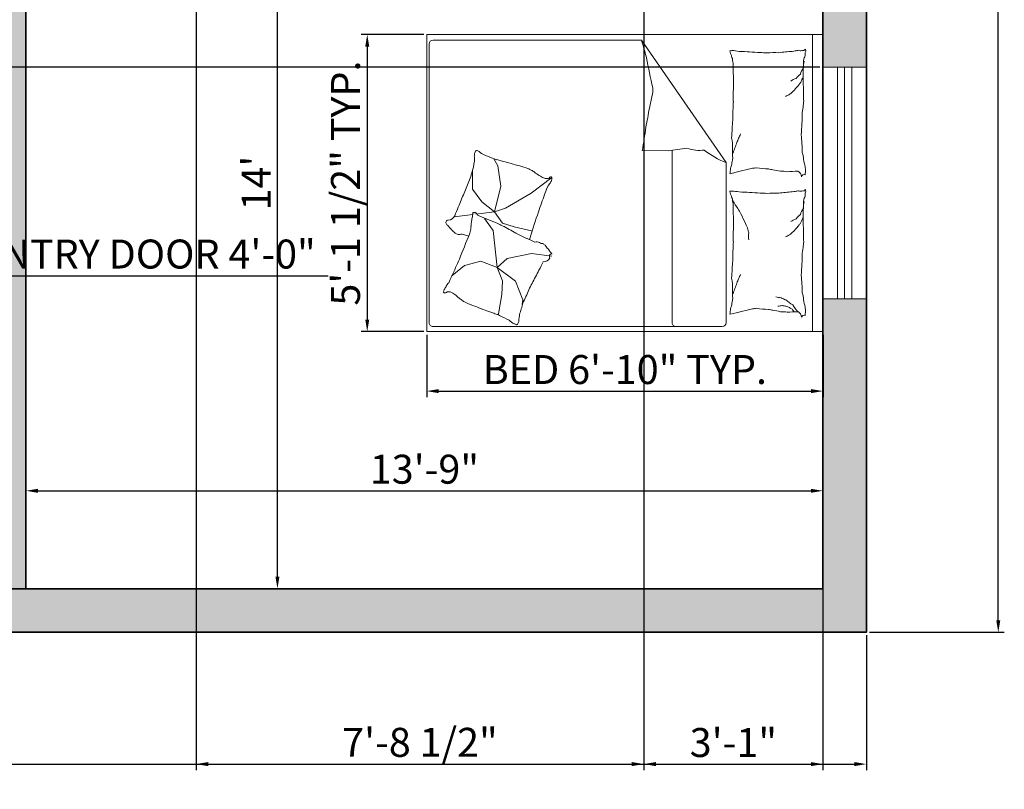
# Model space of a CAD drawing. Units: inches. Extents: x -40 to 424, y -33 to 568.
# Tile 2 of 8: x 209 to 413, y -33 to 127. Entities that reach past the tile are written whole.
import ezdxf

# ---------------------------------------------------------------- set-up
doc = ezdxf.new("R2010")
doc.units = ezdxf.units.IN
for name, color, linetype, lineweight in [('A-ANNO-DIMS', 7, 'Continuous', 18), ('A-FURN', 7, 'Continuous', 18), ('A-GLAZ', 7, 'Continuous', 18), ('A-WALL-PATT', 30, 'Continuous', 13), ('wall', 7, 'Continuous', 35)]:
    doc.layers.add(name, color=color, linetype=linetype, lineweight=lineweight)
doc.styles.add('DIM_FONT', font='SIMPLEX.shx', dxfattribs={"width": 0.8})
doc.styles.get("Standard").update_dxf_attribs({"font": 'arial.ttf'})
doc.dimstyles.new('ISO-25', dxfattribs={"dimtxt": 6, "dimasz": 2.5, "dimexe": 1.25, "dimexo": 0.625, "dimtad": 1, "dimdec": 1, "dimlunit": 3, "dimtxsty": 'Standard', "dimcen": 2.5, "dimadec": 0, "dimazin": 0, "dimtfac": 1, "dimtdec": 1, "dimtmove": 0, "dimatfit": 3, "dimfxl": 1, "dimarcsym": 0})

# ---------------------------------------------------------------- blocks, each defined once
blk = doc.blocks.new('A$C79B528CE')
for p, q in [((1.5, 2), (0, 2)), ((0, 2), (0, 0)), ((1.5, 0), (1.5, 2)), ((1.5, 1.9476), (0, 1.9476)), ((0.6954, 1.5617), (0.6748, 1.6443)), ((1.4047, 1.5617), (1.384, 1.6443)), ((0.7029, 1.5317), (0.6954, 1.5617)), ((1.4122, 1.5317), (1.4047, 1.5617)), ((0.6465, 1.5115), (0.0284, 1.0841)), ((0.6465, 1.5115), (1.4542, 1.5115)), ((1.4742, 1.4915), (1.4742, 0.0322)), ((0.574, 1.3138), (0.5876, 1.2184)), ((1.4542, 1.2389), (0.5847, 1.2389)), ((0.5876, 1.2184), (0.5859, 1.0883)), ((0.0284, 0.0322), (0.0284, 1.0841)), ((0.7224, 0.6316), (0.8016, 0.5276)), ((1.119, 0.6317), (1.1052, 0.5286)), ((0.8016, 0.5276), (0.8767, 0.3973)), ((0.9716, 0.4407), (0.9914, 0.5296)), ((1.1052, 0.5286), (1.131, 0.4065)), ((1.1757, 0.355), (1.2446, 0.4478)), ((1.2446, 0.4478), (1.3392, 0.4856)), ((1.3392, 0.4856), (1.3632, 0.4822)), ((0.9518, 0.3834), (0.9716, 0.4407)), ((1.131, 0.4065), (1.1757, 0.355)), ((0.6632, 0.3597), (0.6272, 0.3397)), ((0.766, 0.3736), (0.6632, 0.3597)), ((0.8945, 0.342), (0.766, 0.3736)), ((0.8767, 0.3973), (0.8945, 0.342)), ((0.8945, 0.342), (0.9518, 0.3834)), ((0.9527, 0.3558), (0.9297, 0.2995)), ((1.1757, 0.355), (0.99, 0.3361)), ((1.1757, 0.355), (1.1448, 0.2725)), ((1.1757, 0.355), (1.2428, 0.3825)), ((1.2428, 0.3825), (1.3116, 0.379)), ((1.3116, 0.379), (1.4097, 0.3619)), ((1.4097, 0.3619), (1.413, 0.3554)), ((0.8945, 0.342), (0.8451, 0.2787)), ((0.8945, 0.342), (0.9063, 0.2478)), ((0.9297, 0.2995), (0.9119, 0.256)), ((0.9401, 0.3), (0.928, 0.2914)), ((0.99, 0.3361), (0.9401, 0.3)), ((0.8451, 0.2787), (0.7799, 0.2313)), ((1.1448, 0.2725), (1.1654, 0.19)), ((0.7799, 0.2313), (0.687, 0.2313)), ((0.9081, 0.2331), (0.92, 0.1385)), ((1.1654, 0.19), (1.219, 0.1274)), ((1.4542, 0.0122), (0.0484, 0.0122)), ((0, 0), (1.5, 0))]:
    blk.add_line(p, q)
for centre, radius, start, end in [((0.0726, 1.9139), 0.00342, 291.7883, 340.436), ((0.0743, 1.9085), 0.00232, 340.436, 101.8931), ((0.0739, 1.9378), 0.0251, 274.3025, 291.7883), ((0.0805, 1.9093), 0.00428, 201.9904, 281.8931), ((0.049, 1.8889), 0.0328, 338.579, 8.1335), ((0.0959, 1.8994), 0.0156, 158.579, 201.9904), ((0.098, 1.9393), 0.0289, 239.3487, 274.3025), ((0.0952, 1.8568), 0.0539, 59.3487, 84.7408), ((0.0953, 1.0829), 0.8208, 84.7408, 88.0921), ((0.1612, 2.0005), 0.0992, 254.0648, 274.2159), ((0.2269, 1.9817), 0.0992, 233.9136, 254.0648), ((0.1856, 0.406), 1.4943, 88.0921, 90.5757), ((0.323, 2.1075), 0.234, 242.7604, 249.1397), ((0.3084, 1.0293), 0.8732, 90.5757, 94.8018), ((0.2874, 1.949), 0.0768, 231.6114, 242.7604), ((0.3125, 2.1919), 0.2897, 267.4614, 274.8018), ((0.3637, 2.0532), 0.1524, 259.8101, 267.4614), ((0.3008, 1.3747), 0.5293, 79.8101, 83.9133), ((0.3945, 0.8466), 1.049, 83.9133, 90), ((0.5954, 1.2129), 0.6827, 90, 97.5469), ((0.6611, 1.6625), 0.2422, 97.5469, 105.744), ((0.5846, 2.2041), 0.3048, 278.4372, 285.744), ((0.6672, 2.0719), 0.1611, 270, 278.4372), ((0.7204, 1.8579), 0.0342, 94.4002, 153.4195), ((0.7086, 2.0011), 0.0904, 258.7276, 270), ((0.7203, 1.9049), 0.0131, 153.4195, 258.7276), ((0.7818, 1.9139), 0.00342, 291.7883, 340.436), ((0.7836, 1.9085), 0.00232, 340.436, 101.8931), ((0.7831, 1.9378), 0.0251, 274.3025, 291.7883), ((0.7897, 1.9093), 0.00428, 201.9904, 281.8931), ((0.7582, 1.8889), 0.0328, 338.579, 8.1335), ((0.8051, 1.8994), 0.0156, 158.579, 201.9904), ((0.8072, 1.9393), 0.0289, 239.3487, 274.3025), ((0.8044, 1.8568), 0.0539, 59.3487, 84.7408), ((0.8046, 1.0829), 0.8208, 84.7408, 88.0921), ((0.8704, 2.0005), 0.0992, 254.0648, 274.2159), ((0.9361, 1.9817), 0.0992, 233.9136, 254.0648), ((0.8948, 0.406), 1.4943, 88.0921, 90.5757), ((1.0323, 2.1075), 0.234, 242.7604, 249.1397), ((1.0177, 1.0293), 0.8732, 90.5757, 94.8018), ((0.9966, 1.949), 0.0768, 231.6114, 242.7604), ((1.0217, 2.1919), 0.2897, 267.4614, 274.8018), ((1.0729, 2.0532), 0.1524, 259.8101, 267.4614), ((1.0101, 1.3747), 0.5293, 79.8101, 83.9133), ((1.1037, 0.8466), 1.049, 83.9133, 90), ((1.3046, 1.2129), 0.6827, 90, 97.5469), ((1.3703, 1.6625), 0.2422, 97.5469, 105.744), ((1.2938, 2.2041), 0.3048, 278.4372, 285.744), ((1.3765, 2.0719), 0.1611, 270, 278.4372), ((1.4296, 1.8579), 0.0342, 94.4002, 153.4195), ((1.4178, 2.0011), 0.0904, 258.7276, 270), ((1.4295, 1.9049), 0.0131, 153.4195, 258.7276), ((-0.1611, 1.8253), 0.246, 8.1335, 12.1095), ((0.279, 1.8867), 0.1983, 187.6809, 192.1095), ((0.9966, 1.8987), 0.9131, 183.3687, 187.6809), ((0.2797, 1.9449), 0.0992, 216.1766, 233.9136), ((0.3154, 1.8961), 0.0992, 198.4397, 216.1766), ((0.5234, 2.1633), 0.3916, 226.1885, 231.6114), ((0.4551, 1.9982), 0.2252, 219.0349, 226.1885), ((1.1818, 1.8735), 0.4918, 180, 186.2324), ((0.5482, 1.8253), 0.246, 8.1335, 12.1095), ((0.9883, 1.8867), 0.1983, 187.6809, 192.1095), ((1.7058, 1.8987), 0.9131, 183.3687, 187.6809), ((0.989, 1.9449), 0.0992, 216.1766, 233.9136), ((1.0247, 1.8961), 0.0992, 198.4397, 216.1766), ((1.2326, 2.1633), 0.3916, 226.1885, 231.6114), ((1.1643, 1.9982), 0.2252, 219.0349, 226.1885), ((1.2401, 1.9123), 0.1399, 314.9024, 332.6012), ((1.3004, 1.9723), 0.1399, 297.2036, 314.9024), ((1.3389, 1.8667), 0.0526, 318.5571, 334.6449), ((1.3333, 1.9167), 0.0899, 306.2641, 318.5571), ((1.891, 1.8735), 0.4918, 180, 186.2324), ((0.3426, 1.8591), 0.0493, 208.3168, 219.0349), ((0.4886, 1.9062), 0.2002, 203.0028, 208.3168), ((0.8939, 1.7858), 0.204, 170.3156, 180), ((1.0518, 1.8591), 0.0493, 208.3168, 219.0349), ((1.1978, 1.9062), 0.2002, 203.0028, 208.3168), ((1.2048, 1.8529), 0.1399, 332.6012, 343.485), ((1.3147, 1.8132), 0.0562, 341.2201, 0), ((1.2793, 1.7719), 0.0915, 0, 14.6851), ((1.18, 1.8895), 0.2056, 338.1851, 341.2201), ((1.2381, 1.8881), 0.1511, 334.6449, 338.1851), ((1.6031, 1.7858), 0.204, 170.3156, 180), ((0.7702, 1.7573), 0.6787, 178.3669, 183.3687), ((0.3686, 1.792), 0.3171, 347.8016, 351.9949), ((1.552, 1.5994), 0.882, 167.8016, 170.3156), ((1.4794, 1.7573), 0.6787, 178.3669, 183.3687), ((1.1897, 1.8023), 0.1399, 343.485, 354.3689), ((1.0778, 1.792), 0.3171, 347.8016, 351.9949), ((2.2613, 1.5994), 0.882, 167.8016, 170.3156), ((1.4559, 1.6447), 1.3652, 176.945, 178.3669), ((0.0204, 1.7556), 0.6588, 351.9949, 357.3351), ((2.1651, 1.6447), 1.3652, 176.945, 178.3669), ((0.7297, 1.7556), 0.6588, 351.9949, 357.3351), ((13.7013, 0.85), 13.6356, 176.49514, 176.94504), ((0.6071, 1.6474), 0.0677, 357.3351, 14.0452), ((14.4105, 0.85), 13.6356, 176.49514, 176.94504), ((1.3164, 1.6474), 0.0677, 357.3351, 14.0452), ((0.3151, 2.8912), 1.4323, 294.3265, 296.4985), ((0.7753, 2.0834), 0.5066, 290.6743, 294.3265), ((0.9799, 1.6796), 0.058, 274.0828, 290.6743), ((1.0172, 1.8969), 0.2721, 266.4448, 274.0828), ((0.4014, 1.5209), 0.3212, 170.0016, 176.4951), ((0.1, 1.5832), 0.0453, 282.869, 297.2841), ((0.1117, 1.6885), 0.1459, 273.574, 282.869), ((0.1384, 2.7103), 1.164, 270.2865, 273.574), ((0.3078, 7.2662), 5.7185, 269.0296, 270.2865), ((0.4895, 4.9065), 3.3622, 267.3904, 269.0296), ((0.5304, 2.7573), 1.2165, 265.3824, 267.3904), ((0.4077, 0.139), 1.4048, 85.3824, 87.2509), ((0.2076, 0.9067), 0.7387, 64.6889, 66.5156), ((0.5669, 1.3138), 0.2301, 87.2509, 101.5586), ((0.2508, 0.888), 0.7387, 66.5156, 68.3423), ((0.2995, 0.8688), 0.7387, 68.3423, 70.572), ((0.3537, 0.8497), 0.7387, 70.572, 72.8018), ((0.5943, 1.6886), 0.1459, 263.5659, 281.5586), ((0.6593, 1.6599), 0.1197, 252.6136, 263.5659), ((0.608, 1.3144), 0.2297, 72.6136, 80.5159), ((1.1107, 1.5209), 0.3212, 170.0016, 176.4951), ((0.8093, 1.5832), 0.0453, 282.869, 297.2841), ((0.8209, 1.6885), 0.1459, 273.574, 282.869), ((0.4519, 2.1618), 0.7286, 302.135, 305.8263), ((0.8476, 2.7103), 1.164, 270.2865, 273.574), ((0.7388, 1.8508), 0.3126, 296.4985, 302.135), ((1.017, 7.2662), 5.7185, 269.0296, 270.2865), ((1.1987, 4.9065), 3.3622, 267.3904, 269.0296), ((1.2397, 2.7573), 1.2165, 265.3824, 267.3904), ((1.1169, 0.139), 1.4048, 85.3824, 87.2509), ((0.9169, 0.9067), 0.7387, 64.6889, 66.5156), ((1.2761, 1.3138), 0.2301, 87.2509, 101.5586), ((0.9601, 0.888), 0.7387, 66.5156, 68.3423), ((1.0087, 0.8688), 0.7387, 68.3423, 70.572), ((1.0629, 0.8497), 0.7387, 70.572, 72.8018), ((1.3035, 1.6886), 0.1459, 263.5659, 281.5586), ((1.3685, 1.6599), 0.1197, 252.6136, 263.5659), ((1.3172, 1.3144), 0.2297, 72.6136, 80.5159), ((0.0623, 1.535), 0.0193, 350.0016, 16.6978), ((0.0815, 1.5304), 0.00132, 16.6978, 97.1204), ((0.1072, 1.4467), 0.0875, 97.1204, 106.2212), ((0.1315, 1.4654), 0.0767, 106.2212, 117.2841), ((0.2944, 1.6407), 0.3751, 320.3555, 339.8512), ((0.6574, 1.2635), 0.2708, 80.5159, 85.9171), ((0.7029, 1.5308), 0.000917, 85.9171, 194.0449), ((0.7716, 1.535), 0.0193, 350.0016, 16.6978), ((0.7908, 1.5304), 0.00132, 16.6978, 97.1204), ((0.8165, 1.4467), 0.0875, 97.1204, 106.2212), ((0.8408, 1.4654), 0.0767, 106.2212, 117.2841), ((1.3666, 1.2635), 0.2708, 80.5159, 85.9171), ((1.4121, 1.5308), 0.000917, 85.9171, 194.0449), ((1.4542, 1.4915), 0.02, 0, 90), ((0.4049, 1.3759), 0.1801, 339.8512, 8.1356), ((1.4542, 1.2589), 0.02, 270, 0), ((-0.4754, 2.8487), 1.8351, 285.9352, 287.7364), ((-0.0634, 1.7415), 0.6574, 282.9255, 285.9352), ((-0.6395, 5.1029), 4.0646, 280.7276, 282.9255), ((0.2775, 1.1989), 0.0581, 262.2696, 280.7276), ((0.3326, 1.3309), 0.1942, 256.8096, 262.2696), ((-0.2025, -1.3253), 2.5158, 76.8096, 78.3259), ((-0.0554, -1.4284), 2.588, 78.3259, 80.505), ((-0.0377, -2.64), 3.7801, 80.505, 82.308), ((0.7246, 0.6267), 0.0063, 166.7192, 233.4208), ((0.7227, 0.6272), 0.00443, 93.9484, 166.7192), ((0.7124, 0.6103), 0.0142, 10.4074, 53.4208), ((0.7249, 0.5964), 0.0352, 69.6548, 93.9484), ((0.6889, 0.6079), 0.0393, 333.1821, 345.4291), ((0.6504, 0.5989), 0.0771, 2.7286, 10.4074), ((0.7122, 0.6019), 0.0153, 345.4291, 2.7286), ((0.7162, 0.5731), 0.0601, 51.4146, 69.6548), ((0.8031, 0.682), 0.0792, 231.4146, 247.2931), ((1.0957, 1.3811), 0.8371, 247.2931, 249.8713), ((1.0012, 0.6426), 0.0774, 313.5224, 324.1064), ((0.9323, 0.7705), 0.2176, 307.2151, 313.5224), ((0.692, 1.1456), 0.6605, 306.2163, 307.2151), ((1.3244, 0.3162), 0.3825, 126.2163, 127.5287), ((1.1299, 0.5924), 0.0452, 127.5287, 134.1274), ((1.0587, 0.6825), 0.0697, 308.8136, 314.1274), ((1.1199, 0.6318), 0.0127, 176.7545, 308.8136), ((1.1115, 0.59), 0.0359, 356.7545, 62.7098), ((0.5455, 0.6678), 0.194, 320.2995, 329.0944), ((0.4099, 0.749), 0.352, 329.0944, 333.1821), ((2.5607, 5.3783), 5.0942, 249.8713, 250.9164), ((1.9234, 3.5362), 3.145, 250.9164, 253.3915), ((1.0928, 0.5526), 0.0458, 157.5838, 188.0492), ((1.0322, 0.5833), 0.0226, 324.1064, 8.0492), ((-0.2306, -2.1858), 3.0972, 62.7098, 63.5853), ((2.1205, 2.3551), 2.0162, 242.5001, 243.5853), ((4.0739, 5.9445), 6.1019, 242.15178, 242.50014), ((2.5804, -0.112), 2.003, 162.1604, 164.7375), ((0.8608, 0.4414), 0.1965, 153.9265, 162.1604), ((0.7571, 0.4922), 0.081, 140.2995, 153.9265), ((2.5307, -0.2643), 1.6868, 152.9116, 154.9471), ((1.0578, 0.6341), 0.1166, 253.3915, 259.2634), ((1.9583, 0.1204), 1.0054, 154.9471, 157.5838), ((-1.4387, -4.647), 5.8383, 62.15178, 62.50792), ((1.0676, -0.068), 0.6236, 62.5079, 69.2514), ((2.3589, -0.3311), 1.5652, 150.064, 152.9116), ((1.2615, 0.0657), 0.43, 69.2514, 77.3748), ((1.4175, 0.4049), 0.063, 77.3748, 93.3881), ((1.4448, 0.5247), 0.0599, 256.9598, 273.3881), ((1.4751, 0.5082), 0.0509, 238.3083, 256.9598), ((1.4772, 0.441), 0.0168, 130.5086, 180.9614), ((1.4694, 0.4587), 0.0058, 180.9614, 238.3083), ((2.2381, -0.0186), 1.6481, 164.7375, 166.159), ((-0.9672, 1.5491), 2.6619, 333.6668, 334.8268), ((1.3928, 0.4743), 0.0755, 310.5086, 333.6668), ((0.4592, 0.4035), 0.1798, 339.2227, 343.6878), ((0.1082, 0.5062), 0.5454, 343.6878, 346.159), ((0.767, 0.4627), 0.2143, 330.064, 337.7645), ((0.895, 0.5261), 0.5454, 339.2919, 341.7631), ((1.2503, 0.4319), 0.1798, 334.8268, 339.2919), ((-1.8615, 1.284), 2.6619, 338.0627, 339.2227), ((2.9572, -0.2212), 1.6481, 160.3416, 161.7631), ((0.6027, 0.2524), 0.0168, 134.9045, 185.3572), ((0.5918, 0.2513), 0.0058, 185.3572, 242.7041), ((0.5376, 0.3177), 0.0755, 314.9045, 338.0627), ((0.9188, 0.234), 0.0231, 107.1867, 157.7645), ((3.2459, -0.4634), 2.003, 157.7645, 160.3416), ((0.6125, 0.2914), 0.0509, 242.7041, 261.3557), ((0.6138, 0.3003), 0.0599, 261.3557, 277.784), ((0.6305, 0.1786), 0.063, 81.7707, 97.784), ((0.5779, -0.1846), 0.43, 73.6473, 81.7707), ((0.5234, -0.3705), 0.6236, 66.9038, 73.6473), ((-1.5222, -5.1672), 5.8383, 66.54766, 66.9038), ((0.8959, 0.2383), 0.00467, 287.1867, 70.6201), ((0.8979, 0.2247), 0.0092, 70.6201, 94.2593), ((0.9057, 0.267), 0.034, 262.0178, 274.2593), ((0.9584, 0.4221), 0.1955, 255.1193, 262.0178), ((0.9073, 0.0507), 0.1794, 75.1193, 82.3216), ((0.959, 0.153), 0.0712, 82.3216, 94.5118), ((0.9779, 0.2893), 0.0663, 261.8784, 274.5118), ((1.0249, 0.332), 0.1166, 248.9957, 261.8784), ((2.2614, 3.1012), 3.145, 246.5205, 248.9957), ((1.9669, -0.1202), 1.0054, 160.6552, 161.9797), ((1.529, 0.1108), 0.1965, 149.5306, 157.7645), ((3.2298, 5.7866), 6.1019, 246.54766, 246.89602), ((1.6266, 2.0287), 2.0162, 246.896, 247.9812), ((-0.2904, -2.7118), 3.0972, 67.1056, 67.9812), ((0.9408, 0.1905), 0.0774, 317.9183, 328.5023), ((0.9875, 0.1619), 0.0226, 328.5023, 12.4451), ((1.0543, 0.1766), 0.0458, 161.9797, 192.4451), ((3.2487, 4.7998), 5.0942, 245.4754, 246.5205), ((1.1772, 0.2819), 0.194, 315.9036, 324.6985), ((1.4053, 0.1288), 0.081, 135.9036, 149.5306), ((0.9005, 0.1084), 0.0359, 1.1504, 67.1056), ((0.9491, 0.1094), 0.0127, 181.1504, 313.2095), ((0.9101, 0.1509), 0.0697, 313.2095, 318.5233), ((0.9962, 0.0748), 0.0452, 131.9246, 138.5233), ((1.2216, -0.1762), 0.3825, 130.6122, 131.9246), ((0.5426, 0.6156), 0.6605, 310.6122, 311.611), ((0.8367, 0.2845), 0.2176, 311.611, 317.9183), ((1.6004, 0.8725), 0.8371, 242.8972, 245.4754), ((1.3069, 0.1689), 0.0792, 227.0187, 242.8972), ((1.2839, 0.1188), 0.0153, 341.0332, 358.3327), ((1.2216, 0.1058), 0.0771, 358.3327, 6.0115), ((1.2895, 0.0928), 0.0142, 6.0115, 49.0249), ((1.2655, 0.1388), 0.0393, 328.7862, 341.0332), ((1.0155, 0.3294), 0.352, 324.6985, 328.7862), ((1.2457, 0.0438), 0.0601, 47.0187, 65.2589), ((1.2864, 0.0526), 0.0352, 65.2589, 89.5525), ((1.3054, 0.0832), 0.00443, 89.5525, 162.3233), ((1.3095, 0.0924), 0.0063, 162.3233, 229.0249), ((0.0484, 0.0322), 0.02, 180, 270), ((1.4542, 0.0322), 0.02, 270, 0)]:
    blk.add_arc(centre, radius, start, end)
at = {"style": 'DIM_FONT', "oblique": -180, "text_generation_flag": 4, "width": 0.8, "flags": 9}
for tag in ['XSIZE', 'YSIZE']:
    blk.add_attdef(tag, (1.5, 2), '', height=0.0005, rotation=180, dxfattribs=at)
blk = doc.blocks.new('*D19')
at = {"layer": 'A-ANNO-DIMS', "color": 0, "lineweight": -2, "transparency": 16777216}
for p, q in [((210, 26.12), (210, 30.54)), ((212.5, 29.29), (372.5, 29.29)), ((375, 26.12), (375, 30.54))]:
    blk.add_line(p, q, dxfattribs=at)
at = {"layer": 'A-ANNO-DIMS', "color": 0, "transparency": 16777216}
for points in [[(212.5, 29.7), (212.5, 28.87), (210, 29.29)], [(372.5, 29.7), (372.5, 28.87), (375, 29.29)]]:
    blk.add_solid(points, dxfattribs=at)
at = {"layer": 'Defpoints', "color": 0, "transparency": 16777216}
for p in [(375, 29.29), (210, 25.5), (375, 25.5)]:
    blk.add_point(p, dxfattribs=at)
at = {"layer": 'A-ANNO-DIMS', "color": 0, "transparency": 16777216, "insert": (292.5, 32.98), "char_height": 6, "attachment_point": 5}
blk.add_mtext('13\'-9"', dxfattribs=at)
blk = doc.blocks.new('*D20')
at = {"layer": 'A-ANNO-DIMS', "color": 0, "lineweight": -2, "transparency": 16777216}
for p, q in [((262.04, 177), (260.82, 177)), ((262.07, 11.5), (262.07, 174.5)), ((262.04, 9), (260.82, 9))]:
    blk.add_line(p, q, dxfattribs=at)
at = {"layer": 'A-ANNO-DIMS', "color": 0, "transparency": 16777216}
for points in [[(261.66, 174.5), (262.49, 174.5), (262.07, 177)], [(261.66, 11.5), (262.49, 11.5), (262.07, 9)]]:
    blk.add_solid(points, dxfattribs=at)
at = {"layer": 'Defpoints', "color": 0, "transparency": 16777216}
for p in [(262.07, 177), (262.66, 177), (262.66, 9)]:
    blk.add_point(p, dxfattribs=at)
at = {"layer": 'A-ANNO-DIMS', "color": 0, "transparency": 16777216, "insert": (258.44, 93), "char_height": 6, "attachment_point": 5, "rotation": 90}
blk.add_mtext("14'", dxfattribs=at)
blk = doc.blocks.new('WIN-48IN')
for p, q in [((0, 0), (0, 9)), ((48, 0), (48, 9)), ((0, 6), (48, 6)), ((0, 4.5), (48, 4.5)), ((0, 3), (48, 3))]:
    blk.add_line(p, q)
blk = doc.blocks.new('*D51')
at = {"layer": 'A-ANNO-DIMS', "color": 0, "lineweight": -2, "transparency": 16777216}
for p, q in [((147, 80.37), (147, 72.55)), ((195, 80.37), (195, 72.55)), ((149.5, 73.8), (192.5, 73.8)), ((195, 73.8), (272.6, 73.8))]:
    blk.add_line(p, q, dxfattribs=at)
at = {"layer": 'A-ANNO-DIMS', "color": 0, "transparency": 16777216}
for points in [[(149.5, 74.22), (149.5, 73.38), (147, 73.8)], [(192.5, 74.22), (192.5, 73.38), (195, 73.8)]]:
    blk.add_solid(points, dxfattribs=at)
at = {"layer": 'Defpoints', "color": 0, "transparency": 16777216}
for p in [(147, 81), (195, 81), (195, 73.8)]:
    blk.add_point(p, dxfattribs=at)
at = {"layer": 'A-ANNO-DIMS', "color": 0, "transparency": 16777216, "insert": (235.05, 77.53), "char_height": 6, "attachment_point": 5}
blk.add_mtext('ENTRY DOOR 4\'-0"', dxfattribs=at)
blk = doc.blocks.new('*D57')
at = {"layer": 'A-ANNO-DIMS', "color": 0, "lineweight": -2, "transparency": 16777216}
for p, q in [((292.97, 61.61), (292.97, 48.68)), ((375.02, 61.61), (375.02, 48.68)), ((295.47, 49.93), (372.52, 49.93))]:
    blk.add_line(p, q, dxfattribs=at)
at = {"layer": 'A-ANNO-DIMS', "color": 0, "transparency": 16777216}
for points in [[(295.47, 50.35), (295.47, 49.51), (292.97, 49.93)], [(372.52, 50.35), (372.52, 49.51), (375.02, 49.93)]]:
    blk.add_solid(points, dxfattribs=at)
at = {"layer": 'Defpoints', "color": 0, "transparency": 16777216}
for p in [(292.97, 62.24), (375.02, 62.24), (375.02, 49.93)]:
    blk.add_point(p, dxfattribs=at)
at = {"layer": 'A-ANNO-DIMS', "color": 0, "transparency": 16777216, "insert": (334, 53.62), "char_height": 6, "attachment_point": 5}
blk.add_mtext('BED 6\'-10" TYP.', dxfattribs=at)
blk = doc.blocks.new('*D58')
at = {"layer": 'A-ANNO-DIMS', "color": 0, "lineweight": -2, "transparency": 16777216}
for p, q in [((292.35, 123.76), (279.41, 123.76)), ((280.66, 121.26), (280.66, 64.74)), ((292.35, 62.24), (279.41, 62.24))]:
    blk.add_line(p, q, dxfattribs=at)
at = {"layer": 'A-ANNO-DIMS', "color": 0, "transparency": 16777216}
for points in [[(280.25, 121.26), (281.08, 121.26), (280.66, 123.76)], [(280.25, 64.74), (281.08, 64.74), (280.66, 62.24)]]:
    blk.add_solid(points, dxfattribs=at)
at = {"layer": 'Defpoints', "color": 0, "transparency": 16777216}
for p in [(292.97, 123.76), (280.66, 62.24), (292.97, 62.24)]:
    blk.add_point(p, dxfattribs=at)
at = {"layer": 'A-ANNO-DIMS', "color": 0, "transparency": 16777216, "insert": (276.94, 93), "char_height": 6, "attachment_point": 5, "rotation": 90}
blk.add_mtext('5\'-1 1/2" TYP.', dxfattribs=at)
blk = doc.blocks.new('*D79')
at = {"layer": 'A-ANNO-DIMS', "color": 0, "lineweight": -2, "transparency": 16777216}
for p, q in [((0, -0.62), (0, -28.55)), ((384, -0.62), (384, -28.55)), ((2.5, -27.3), (381.5, -27.3))]:
    blk.add_line(p, q, dxfattribs=at)
at = {"layer": 'A-ANNO-DIMS', "color": 0, "transparency": 16777216}
for points in [[(2.5, -26.88), (2.5, -27.72), (0, -27.3)], [(381.5, -26.88), (381.5, -27.72), (384, -27.3)]]:
    blk.add_solid(points, dxfattribs=at)
at = {"layer": 'Defpoints', "color": 0, "transparency": 16777216}
for p in [(0, 0), (384, 0), (384, -27.3)]:
    blk.add_point(p, dxfattribs=at)
at = {"layer": 'A-ANNO-DIMS', "color": 0, "transparency": 16777216, "insert": (192, -23.61), "char_height": 6, "attachment_point": 5}
blk.add_mtext('32\'-0"', dxfattribs=at)
blk = doc.blocks.new('*D80')
at = {"layer": 'A-ANNO-DIMS', "color": 0, "lineweight": -2, "transparency": 16777216}
for p, q in [((384.63, 528), (412.55, 528)), ((411.3, 2.5), (411.3, 525.5)), ((384.63, 0), (412.55, 0))]:
    blk.add_line(p, q, dxfattribs=at)
at = {"layer": 'A-ANNO-DIMS', "color": 0, "transparency": 16777216}
for points in [[(410.88, 525.5), (411.72, 525.5), (411.3, 528)], [(410.88, 2.5), (411.72, 2.5), (411.3, 0)]]:
    blk.add_solid(points, dxfattribs=at)
at = {"layer": 'Defpoints', "color": 0, "transparency": 16777216}
for p in [(384, 528), (411.3, 528), (384, 0)]:
    blk.add_point(p, dxfattribs=at)
at = {"layer": 'A-ANNO-DIMS', "color": 0, "transparency": 16777216, "insert": (407.61, 264), "char_height": 6, "attachment_point": 5, "rotation": 90}
blk.add_mtext('44\'-0"', dxfattribs=at)
blk = doc.blocks.new('*D87')
at = {"layer": 'A-ANNO-DIMS', "color": 0, "lineweight": -2, "transparency": 16777216}
for p, q in [((374.38, 177), (-28.55, 177)), ((-27.3, 119.5), (-27.3, 174.5)), ((374.38, 117), (-28.55, 117))]:
    blk.add_line(p, q, dxfattribs=at)
at = {"layer": 'A-ANNO-DIMS', "color": 0, "transparency": 16777216}
for points in [[(-27.72, 174.5), (-26.88, 174.5), (-27.3, 177)], [(-27.72, 119.5), (-26.88, 119.5), (-27.3, 117)]]:
    blk.add_solid(points, dxfattribs=at)
at = {"layer": 'Defpoints', "color": 0, "transparency": 16777216}
for p in [(-27.3, 177), (375, 177), (375, 117)]:
    blk.add_point(p, dxfattribs=at)
at = {"layer": 'A-ANNO-DIMS', "color": 0, "transparency": 16777216, "insert": (-30.99, 147), "char_height": 6, "attachment_point": 5, "rotation": 90}
blk.add_mtext('5\'-0"', dxfattribs=at)
blk = doc.blocks.new('*D95')
at = {"layer": 'A-ANNO-DIMS', "color": 0, "lineweight": -2, "transparency": 16777216}
for p, q in [((375, 333.88), (375, -28.55)), ((337.92, 320.88), (337.92, -28.55)), ((340.42, -27.3), (372.5, -27.3))]:
    blk.add_line(p, q, dxfattribs=at)
at = {"layer": 'A-ANNO-DIMS', "color": 0, "transparency": 16777216}
for points in [[(340.42, -26.88), (340.42, -27.72), (337.92, -27.3)], [(372.5, -26.88), (372.5, -27.72), (375, -27.3)]]:
    blk.add_solid(points, dxfattribs=at)
at = {"layer": 'Defpoints', "color": 0, "transparency": 16777216}
for p in [(375, 334.5), (337.92, 321.5), (375, -27.3)]:
    blk.add_point(p, dxfattribs=at)
at = {"layer": 'A-ANNO-DIMS', "color": 0, "transparency": 16777216, "insert": (356.46, -23.61), "char_height": 6, "attachment_point": 5}
blk.add_mtext('3\'-1"', dxfattribs=at)
blk = doc.blocks.new('*D96')
at = {"layer": 'A-ANNO-DIMS', "color": 0, "lineweight": -2, "transparency": 16777216}
for p, q in [((245.23, 320.88), (245.23, -28.55)), ((337.92, 320.88), (337.92, -28.55)), ((247.73, -27.3), (335.42, -27.3))]:
    blk.add_line(p, q, dxfattribs=at)
at = {"layer": 'A-ANNO-DIMS', "color": 0, "transparency": 16777216}
for points in [[(247.73, -26.88), (247.73, -27.72), (245.23, -27.3)], [(335.42, -26.88), (335.42, -27.72), (337.92, -27.3)]]:
    blk.add_solid(points, dxfattribs=at)
at = {"layer": 'Defpoints', "color": 0, "transparency": 16777216}
for p in [(245.23, 321.5), (337.92, 321.5), (337.92, -27.3)]:
    blk.add_point(p, dxfattribs=at)
at = {"layer": 'A-ANNO-DIMS', "color": 0, "transparency": 16777216, "insert": (291.58, -23.57), "char_height": 6, "attachment_point": 5}
blk.add_mtext('7\'-8 1/2"', dxfattribs=at)

msp = doc.modelspace()

# ---------------------------------------------------------------- hatches: boundary and pattern name
at = {"layer": 'A-WALL-PATT'}
h = msp.add_hatch(color=256, dxfattribs=at)
h.dxf.hatch_style = 1
h.paths.add_polyline_path([(9, 399), (0, 399), (0, 351), (9, 351)])
h.paths.add_polyline_path([(9, 303), (0, 303), (0, 210), (9, 210)])
h.paths.add_polyline_path([(9, 150), (0, 150), (0, 0), (384, 0), (384, 69), (375, 69), (375, 62.24), (375, 9), (9, 9)])
h.paths.add_polyline_path([(210, 177), (216, 177), (216, 186), (210, 186), (210, 216), (201, 216), (201, 90), (195, 90), (195, 81), (201, 81), (201, 9), (210, 9)])
h.paths.add_polyline_path([(384, 216), (375, 216), (375, 117), (384, 117)])
h.paths.add_polyline_path([(384, 298.5), (375, 298.5), (375, 279), (375, 240), (384, 240)])
h.paths.add_polyline_path([(384, 417), (375, 417), (375, 334.5), (384, 334.5)])
h.paths.add_polyline_path([(384, 528), (216, 528), (216, 519), (375, 519), (375, 465), (384, 465)])
h.paths.add_polyline_path([(192, 528), (0, 528), (0, 511.5), (9, 511.5), (9, 519), (192, 519)])
h.paths.add_polyline_path([(9, 487.5), (0, 487.5), (0, 447), (9, 447)])
h.paths.add_polyline_path([(111, 480), (9, 480), (9, 471), (111, 471)])
h.paths.add_polyline_path([(174, 519), (165, 519), (165, 354), (174, 354)])
h.paths.add_polyline_path([(243, 426), (237.86, 426), (234, 426), (234, 420), (174, 420), (174, 411), (234, 411), (234, 405), (239.14, 405), (243, 405)])
h.paths.add_polyline_path([(243, 519), (234, 519), (234, 460.14, -0.031638), (237.86, 460.2), (237.86, 462), (243, 462)])
h.paths.add_polyline_path([(243, 369), (234, 369), (234, 354), (375, 354), (375, 363), (243, 363)])
h.paths.add_polyline_path([(375, 279), (195, 279), (195, 270), (201, 270), (201, 264), (210, 264), (210, 270), (375, 270)])
h.paths.add_polyline_path([(291, 270), (282, 270), (282, 222), (286.29, 222), (291, 222)])
h.paths.add_polyline_path([(375, 186), (291, 186), (291, 192), (282, 192), (282, 186), (252, 186), (252, 180.86), (252, 177), (375, 177)])
h.paths.add_polyline_path([(147, 279), (9, 279), (9, 270), (147, 270)])

# ---------------------------------------------------------------- linework, layer by layer
at = {"layer": 'wall'}
for p, q in [((375, 9), (375, 519)), ((210, 177), (210, 9)), ((9, 9), (375, 9))]:
    msp.add_line(p, q, dxfattribs=at)
msp.add_lwpolyline([(0, 0), (384, 0), (384, 528), (0, 528)], close=True, dxfattribs=at)

# ---------------------------------------------------------------- block references
at = {"layer": 'A-FURN', "xscale": 41.01472337562348, "yscale": 41.01472337562348, "zscale": 41.01472337562348, "rotation": 270}
msp.add_blockref('A$C79B528CE', (292.97, 123.76), dxfattribs=at)
at = {"layer": 'A-GLAZ', "rotation": 90.00000000000003}
msp.add_blockref('WIN-48IN', (384, 69), dxfattribs=at)

# ---------------------------------------------------------------- dimensions: what is measured, and where the dimension line sits
at = {"layer": 'A-ANNO-DIMS'}
for base, p1, p2, override, picture, middle in [((411.3, 528), (384, 0), (384, 528), {"dimdec": 1, "dimlfac": 1, "dimrnd": 0, "dimzin": 1, "dimdsep": 46, "dimlunit": 4, "dimfrac": 2}, '*D80', (407.61, 264)), ((-27.3, 177), (375, 117), (375, 177), {"dimdec": 1, "dimlfac": 1, "dimrnd": 0, "dimzin": 1, "dimdsep": 46, "dimlunit": 4, "dimfrac": 2}, '*D87', (-30.99, 147)), ((262.07, 177), (262.66, 9), (262.66, 177), {"dimclrd": 0, "dimclre": 0, "dimclrt": 0}, '*D20', (258.44, 93))]:
    dim = msp.add_linear_dim(base=base, p1=p1, p2=p2, angle=90, dimstyle='ISO-25', override=override, dxfattribs=at)
    dim.commit()
    dim.dimension.update_dxf_attribs({"geometry": picture, "text_midpoint": middle})
for base, p1, p2, override, picture, middle in [((375, -27.3), (337.92, 321.5), (375, 334.5), {"dimdec": 1, "dimlfac": 1, "dimrnd": 0, "dimzin": 1, "dimdsep": 46, "dimlunit": 4, "dimfrac": 2}, '*D95', (356.46, -23.61)), ((337.92, -27.3), (245.23, 321.5), (337.92, 321.5), {"dimdec": 1, "dimlfac": 1, "dimrnd": 0, "dimzin": 1, "dimdsep": 46, "dimlunit": 4, "dimfrac": 2}, '*D96', (291.58, -23.57)), ((375, 29.29), (210, 25.5), (375, 25.5), {"dimclrd": 0, "dimclre": 0, "dimclrt": 0}, '*D19', (292.5, 32.98)), ((384, -27.3), (0, 0), (384, 0), {"dimdec": 1, "dimlfac": 1, "dimrnd": 0, "dimzin": 1, "dimdsep": 46, "dimlunit": 4, "dimfrac": 2}, '*D79', (192, -23.61))]:
    dim = msp.add_linear_dim(base=base, p1=p1, p2=p2, dimstyle='ISO-25', override=override, dxfattribs=at)
    dim.commit()
    dim.dimension.update_dxf_attribs({"geometry": picture, "text_midpoint": middle})
dim = msp.add_linear_dim(base=(280.66, 62.24), p1=(292.97, 123.76), p2=(292.97, 62.24), angle=270, text='<> TYP.', dimstyle='ISO-25', override={"dimdec": 1, "dimlfac": 1, "dimrnd": 0, "dimzin": 1, "dimdsep": 46, "dimlunit": 4, "dimfrac": 2}, dxfattribs=at)
dim.commit()
dim.dimension.update_dxf_attribs({"geometry": '*D58', "text_midpoint": (276.94, 93)})
for base, p1, p2, text, picture, middle in [((195, 73.8), (147, 81), (195, 81), 'ENTRY DOOR <>', '*D51', (235.05, 77.53)), ((375.0205, 49.9315), (292.9706, 62.239), (375.0205, 62.239), 'BED <> TYP.', '*D57', (333.9955, 53.6199))]:
    dim = msp.add_linear_dim(base=base, p1=p1, p2=p2, text=text, dimstyle='ISO-25', override={"dimdec": 1, "dimlfac": 1, "dimrnd": 0, "dimzin": 1, "dimdsep": 46, "dimlunit": 4, "dimfrac": 2}, dxfattribs=at)
    dim.commit()
    dim.dimension.update_dxf_attribs({"geometry": picture, "text_midpoint": middle})

doc.saveas('drawing.dxf')
